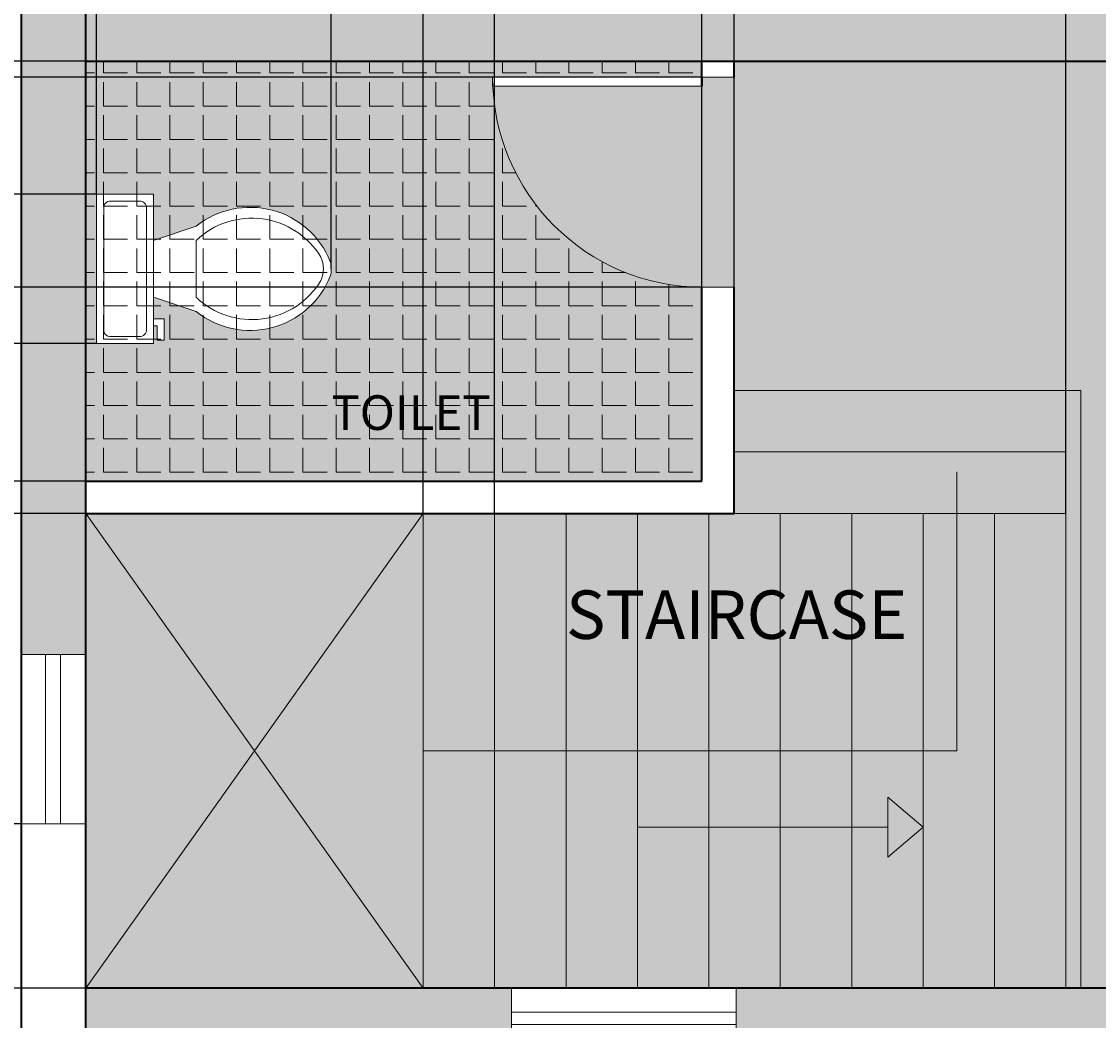
# Model space of a CAD drawing. Units: millimetres. Extents: x -229 to 16545, y -10488 to 4272.
# Tile 3 of 29: x 2016 to 5862, y -4633 to -1067. Entities that reach past the tile are written whole.
import ezdxf

# ---------------------------------------------------------------- set-up
doc = ezdxf.new("R2010")
doc.units = ezdxf.units.MM
for name, color, linetype, lineweight in [('A-ANNO-DIMS', 2, 'Continuous', 18), ('A-ANNO-SYMB', 7, 'Continuous', 18), ('A-AREA-IDEN', 7, 'Continuous', 18), ('A-DOOR', 4, 'Continuous', 18), ('A-FLOR-FIXT', 8, 'Continuous', 18), ('A-FLOR-PATT-TILE', 8, 'Continuous', 13), ('A-FLOR-STRS', 7, 'Continuous', 18), ('A-GLAZ', 4, 'Continuous', 18), ('A-WALL', 7, 'Continuous', 35)]:
    doc.layers.add(name, color=color, linetype=linetype, lineweight=lineweight)
for name, color, linetype, lineweight, true_color in [('A-FLOR-PATT', 254, 'Continuous', 13, 0xfeeab9), ('A-FLOR-STRS-PATT', 51, 'Continuous', 13, 0xf8f6b0), ('A-WALL-PATT', 18, 'Continuous', 13, 0x000000)]:
    doc.layers.add(name, color=color, linetype=linetype, lineweight=lineweight, true_color=true_color)
doc.styles.get("Standard").update_dxf_attribs({"font": 'arial.ttf'})
doc.dimstyles.get("Standard").update_dxf_attribs({"dimtxt": 0.18, "dimasz": 0.18, "dimexe": 0.18, "dimexo": 0.0625, "dimgap": 0.09, "dimtad": 0, "dimtih": 1, "dimtoh": 1, "dimdec": 4, "dimzin": 0, "dimdsep": 46, "dimtxsty": 'Standard', "dimcen": 0.09, "dimadec": 0, "dimazin": 0, "dimtfac": 1, "dimtdec": 4, "dimtofl": 0, "dimtmove": 0, "dimatfit": 3, "dimfxl": 1, "dimtolj": 1, "dimtzin": 0, "dimarcsym": 0})

# ---------------------------------------------------------------- blocks, each defined once
blk = doc.blocks.new('*U13')
at = {"transparency": 33554687}
for p, q in [((0, 0), (0, -6)), ((-40, 0), (-40, -6))]:
    blk.add_line(p, q, dxfattribs=at)
blk.add_lwpolyline([(0, 0), (0, 40), (-1.75, 40), (-1.75, 0)], close=True, dxfattribs=at)
blk.add_arc((0, 0), 40, 90, 180, dxfattribs=at)
blk = doc.blocks.new('*U16')
for p, q in [((9.5, -6), (9.5, -2)), ((-10, -8.5), (-8, -8.5)), ((-10, -9.5), (-10, -8.5)), ((-8, -8.5), (-8, -8)), ((-7, -8), (-7, -9.5)), ((-4, -8), (-6, -14)), ((4, -8), (6, -14)), ((-7, -9.5), (-10, -9.5)), ((4, -14), (-4, -14))]:
    blk.add_line(p, q)
blk.add_lwpolyline([(10.5, -8), (10.5, 0), (-10.5, 0), (-10.5, -8)], close=True)
for points in [[(8.5, -1), (-8.5, -1)], [(-9.5, -2), (-9.5, -6)], [(-8.5, -7), (8.5, -7)]]:
    blk.add_lwpolyline(points)
for centre, radius, start, end in [((-8.62, -1.88), 0.884, 81.8699, 188.1301), ((8.62, -1.88), 0.884, 351.8699, 98.1301), ((-8.62, -6.12), 0.884, 171.8699, 278.1301), ((8.62, -6.12), 0.884, 261.8699, 8.1301), ((3.52, -21.58), 12.17, 141.4691, 247.9714), ((4.2, -21.82), 11.33, 136.3677, 238.9468), ((-3.52, -21.58), 12.17, 292.0284, 38.5307), ((-4.2, -21.82), 11.33, 301.053, 43.6321), ((0, -27.88), 4, 245.7318, 294.2682), ((0, -29), 4, 254.8605, 285.1395)]:
    blk.add_arc(centre, radius, start, end)
blk = doc.blocks.new('WIN-802')
at = {"transparency": 33554687}
for p, q in [((0, 145), (0, 230)), ((802.3, 145), (802.3, 230)), ((0, 100.7), (0, 0)), ((802.3, 100.7), (802.3, 0))]:
    blk.add_line(p, q, dxfattribs=at)
blk.add_lwpolyline([(0, 145), (802.3, 145), (802.3, 100.7), (0, 100.7)], close=True, dxfattribs=at)
blk = doc.blocks.new('*D54')
at = {"layer": 'A-ANNO-DIMS', "color": 0, "lineweight": -2, "transparency": 16777216}
for p, q in [((2245.933029, -2708.209552), (2245.933029, 4271.65929)), ((2246.113029, 4271.47929), (3345.573029, 4271.47929)), ((4445.753029, 4271.47929), (3346.293029, 4271.47929)), ((4445.933029, -2708.209552), (4445.933029, 4271.65929))]:
    blk.add_line(p, q, dxfattribs=at)
at = {"layer": 'A-ANNO-DIMS', "color": 0, "transparency": 16777216}
for points in [[(2246.113029, 4271.50929), (2246.113029, 4271.44929), (2245.933029, 4271.47929)], [(4445.753029, 4271.50929), (4445.753029, 4271.44929), (4445.933029, 4271.47929)]]:
    blk.add_solid(points, dxfattribs=at)
at = {"layer": 'Defpoints', "color": 0, "transparency": 16777216}
for p in [(4445.933029, 4271.47929), (2245.933029, -2708.272052), (4445.933029, -2708.272052)]:
    blk.add_point(p, dxfattribs=at)
at = {"layer": 'A-ANNO-DIMS', "color": 0, "transparency": 16777216, "insert": (3345.933029, 4271.47929), "char_height": 0.18, "attachment_point": 5}
blk.add_mtext('\\A1;2200', dxfattribs=at)
blk = doc.blocks.new('*D55')
at = {"layer": 'A-ANNO-DIMS', "color": 0, "lineweight": -2, "transparency": 16777216}
for p, q in [((4445.9, -1208.3), (-228.8, -1208.3)), ((-228.7, -1208.5), (-228.7, -1958.1)), ((-228.7, -2708.1), (-228.7, -1958.5)), ((4445.9, -2708.3), (-228.8, -2708.3))]:
    blk.add_line(p, q, dxfattribs=at)
at = {"layer": 'A-ANNO-DIMS', "color": 0, "transparency": 16777216}
for points in [[(-228.7, -1208.5), (-228.6, -1208.5), (-228.7, -1208.3)], [(-228.7, -2708.1), (-228.6, -2708.1), (-228.7, -2708.3)]]:
    blk.add_solid(points, dxfattribs=at)
at = {"layer": 'Defpoints', "color": 0, "transparency": 16777216}
for p in [(4445.9, -1208.3), (-228.7, -2708.3), (4445.9, -2708.3)]:
    blk.add_point(p, dxfattribs=at)
at = {"layer": 'A-ANNO-DIMS', "color": 0, "transparency": 16777216, "insert": (-228.7, -1958.3), "char_height": 0.18, "attachment_point": 5}
blk.add_mtext('\\A1;1500', dxfattribs=at)
blk = doc.blocks.new('*D56')
at = {"layer": 'A-ANNO-DIMS', "color": 0, "lineweight": -2, "transparency": 16777216}
for p, q in [((2245.9, -2823.3), (-228.8, -2823.3)), ((-228.7, -2823.5), (-228.7, -3670.6)), ((-228.7, -4518.1), (-228.7, -3671)), ((2245.9, -4518.3), (-228.8, -4518.3))]:
    blk.add_line(p, q, dxfattribs=at)
at = {"layer": 'A-ANNO-DIMS', "color": 0, "transparency": 16777216}
for points in [[(-228.7, -2823.5), (-228.6, -2823.5), (-228.7, -2823.3)], [(-228.7, -4518.1), (-228.6, -4518.1), (-228.7, -4518.3)]]:
    blk.add_solid(points, dxfattribs=at)
at = {"layer": 'Defpoints', "color": 0, "transparency": 16777216}
for p in [(2245.9, -2823.3), (-228.7, -4518.3), (2245.9, -4518.3)]:
    blk.add_point(p, dxfattribs=at)
at = {"layer": 'A-ANNO-DIMS', "color": 0, "transparency": 16777216, "insert": (-228.7, -3670.8), "char_height": 0.18, "attachment_point": 5}
blk.add_mtext('\\A1;1695', dxfattribs=at)
blk = doc.blocks.new('*D81')
at = {"layer": 'A-ANNO-DIMS', "color": 0, "lineweight": -2, "transparency": 16777216}
for p, q in [((2245.9, -2823.2), (2245.9, 4271.7)), ((2246.1, 4271.5), (2847.7, 4271.5)), ((3450.2, 4271.5), (2848.6, 4271.5)), ((3450.4, -2823.2), (3450.4, 4271.7))]:
    blk.add_line(p, q, dxfattribs=at)
at = {"layer": 'A-ANNO-DIMS', "color": 0, "transparency": 16777216}
for points in [[(2246.1, 4271.5), (2246.1, 4271.4), (2245.9, 4271.5)], [(3450.2, 4271.5), (3450.2, 4271.4), (3450.4, 4271.5)]]:
    blk.add_solid(points, dxfattribs=at)
at = {"layer": 'Defpoints', "color": 0, "transparency": 16777216}
for p in [(3450.4, 4271.5), (2245.9, -2823.3), (3450.4, -2823.3)]:
    blk.add_point(p, dxfattribs=at)
at = {"layer": 'A-ANNO-DIMS', "color": 0, "transparency": 16777216, "insert": (2848.2, 4271.5), "char_height": 0.18, "attachment_point": 5}
blk.add_mtext('\\A1;1204.5', dxfattribs=at)
blk = doc.blocks.new('*D82')
at = {"layer": 'A-ANNO-DIMS', "color": 0, "lineweight": -2, "transparency": 16777216}
for p, q in [((3450.4, -2823.2), (3450.4, 4271.7)), ((3450.6, 4271.5), (3577.5, 4271.5)), ((3705.3, 4271.5), (3578.4, 4271.5)), ((3705.5, -2823.2), (3705.5, 4271.7))]:
    blk.add_line(p, q, dxfattribs=at)
at = {"layer": 'A-ANNO-DIMS', "color": 0, "transparency": 16777216}
for points in [[(3450.6, 4271.5), (3450.6, 4271.4), (3450.4, 4271.5)], [(3705.3, 4271.5), (3705.3, 4271.4), (3705.5, 4271.5)]]:
    blk.add_solid(points, dxfattribs=at)
at = {"layer": 'Defpoints', "color": 0, "transparency": 16777216}
for p in [(3705.5, 4271.5), (3450.4, -2823.3), (3705.5, -2823.3)]:
    blk.add_point(p, dxfattribs=at)
at = {"layer": 'A-ANNO-DIMS', "color": 0, "transparency": 16777216, "insert": (3577.9, 4271.5), "char_height": 0.18, "attachment_point": 5}
blk.add_mtext('\\A1;255.06', dxfattribs=at)
blk = doc.blocks.new('*D83')
at = {"layer": 'A-ANNO-DIMS', "color": 0, "lineweight": -2, "transparency": 16777216}
for p, q in [((4448.4, -1265.8), (-228.8, -1265.8)), ((-228.7, -1266), (-228.7, -1640.6)), ((-228.7, -2015.6), (-228.7, -1641)), ((4445.9, -2015.8), (-228.8, -2015.8))]:
    blk.add_line(p, q, dxfattribs=at)
at = {"layer": 'A-ANNO-DIMS', "color": 0, "transparency": 16777216}
for points in [[(-228.7, -1266), (-228.6, -1266), (-228.7, -1265.8)], [(-228.7, -2015.6), (-228.6, -2015.6), (-228.7, -2015.8)]]:
    blk.add_solid(points, dxfattribs=at)
at = {"layer": 'Defpoints', "color": 0, "transparency": 16777216}
for p in [(4448.4, -1265.8), (-228.7, -2015.8), (4445.9, -2015.8)]:
    blk.add_point(p, dxfattribs=at)
at = {"layer": 'A-ANNO-DIMS', "color": 0, "transparency": 16777216, "insert": (-228.7, -1640.8), "char_height": 0.18, "attachment_point": 5}
blk.add_mtext('\\A1;750', dxfattribs=at)
blk = doc.blocks.new('*D84')
at = {"layer": 'A-ANNO-DIMS', "color": 0, "lineweight": -2, "transparency": 16777216}
for p, q in [((4445.9, -2708.2), (4445.9, 4271.7)), ((4446.1, 4271.5), (4503.2, 4271.5)), ((4560.8, 4271.5), (4503.7, 4271.5)), ((4560.9, -2823.2), (4560.9, 4271.7))]:
    blk.add_line(p, q, dxfattribs=at)
at = {"layer": 'A-ANNO-DIMS', "color": 0, "transparency": 16777216}
for points in [[(4446.1, 4271.5), (4446.1, 4271.4), (4445.9, 4271.5)], [(4560.8, 4271.5), (4560.8, 4271.4), (4560.9, 4271.5)]]:
    blk.add_solid(points, dxfattribs=at)
at = {"layer": 'Defpoints', "color": 0, "transparency": 16777216}
for p in [(4560.9, 4271.5), (4445.9, -2708.3), (4560.9, -2823.3)]:
    blk.add_point(p, dxfattribs=at)
at = {"layer": 'A-ANNO-DIMS', "color": 0, "transparency": 16777216, "insert": (4503.4, 4271.5), "char_height": 0.18, "attachment_point": 5}
blk.add_mtext('\\A1;115', dxfattribs=at)
blk = doc.blocks.new('*D88')
at = {"layer": 'A-ANNO-DIMS', "color": 0, "lineweight": -2, "transparency": 16777216}
for p, q in [((2015.9, -3931), (-228.8, -3931)), ((-228.7, -3931.2), (-228.7, -4224.5)), ((-228.7, -4518.1), (-228.7, -4224.8)), ((2245.9, -4518.3), (-228.8, -4518.3))]:
    blk.add_line(p, q, dxfattribs=at)
at = {"layer": 'A-ANNO-DIMS', "color": 0, "transparency": 16777216}
for points in [[(-228.7, -3931.2), (-228.6, -3931.2), (-228.7, -3931)], [(-228.7, -4518.1), (-228.6, -4518.1), (-228.7, -4518.3)]]:
    blk.add_solid(points, dxfattribs=at)
at = {"layer": 'Defpoints', "color": 0, "transparency": 16777216}
for p in [(2015.9, -3931), (-228.7, -4518.3), (2245.9, -4518.3)]:
    blk.add_point(p, dxfattribs=at)
at = {"layer": 'A-ANNO-DIMS', "color": 0, "transparency": 16777216, "insert": (-228.7, -4224.7), "char_height": 0.18, "attachment_point": 5}
blk.add_mtext('\\A1;587.2', dxfattribs=at)
blk = doc.blocks.new('*D93')
at = {"layer": 'A-ANNO-DIMS', "color": 0, "lineweight": -2, "transparency": 16777216}
for p, q in [((2284, -1683.4), (2284, 4271.7)), ((2284.2, 4271.5), (2702.7, 4271.5)), ((3122, 4271.5), (2703.5, 4271.5)), ((3122.2, -1950.1), (3122.2, 4271.7))]:
    blk.add_line(p, q, dxfattribs=at)
at = {"layer": 'A-ANNO-DIMS', "color": 0, "transparency": 16777216}
for points in [[(2284.2, 4271.5), (2284.2, 4271.4), (2284, 4271.5)], [(3122, 4271.5), (3122, 4271.4), (3122.2, 4271.5)]]:
    blk.add_solid(points, dxfattribs=at)
at = {"layer": 'Defpoints', "color": 0, "transparency": 16777216}
for p in [(3122.2, 4271.5), (2284, -1683.5), (3122.2, -1950.2)]:
    blk.add_point(p, dxfattribs=at)
at = {"layer": 'A-ANNO-DIMS', "color": 0, "transparency": 16777216, "insert": (2703.1, 4271.5), "char_height": 0.18, "attachment_point": 5}
blk.add_mtext('\\A1;838.2', dxfattribs=at)
blk = doc.blocks.new('*D94')
at = {"layer": 'A-ANNO-DIMS', "color": 0, "lineweight": -2, "transparency": 16777216}
for p, q in [((2283.9, -1683.5), (-228.8, -1683.5)), ((-228.7, -1683.7), (-228.7, -1950)), ((-228.7, -2216.7), (-228.7, -1950.4)), ((2283.9, -2216.9), (-228.8, -2216.9))]:
    blk.add_line(p, q, dxfattribs=at)
at = {"layer": 'A-ANNO-DIMS', "color": 0, "transparency": 16777216}
for points in [[(-228.7, -1683.7), (-228.6, -1683.7), (-228.7, -1683.5)], [(-228.7, -2216.7), (-228.6, -2216.7), (-228.7, -2216.9)]]:
    blk.add_solid(points, dxfattribs=at)
at = {"layer": 'Defpoints', "color": 0, "transparency": 16777216}
for p in [(2284, -1683.5), (-228.7, -2216.9), (2284, -2216.9)]:
    blk.add_point(p, dxfattribs=at)
at = {"layer": 'A-ANNO-DIMS', "color": 0, "transparency": 16777216, "insert": (-228.7, -1950.2), "char_height": 0.18, "attachment_point": 5}
blk.add_mtext('\\A1;533.4', dxfattribs=at)
blk = doc.blocks.new('*D97')
at = {"layer": 'A-ANNO-DIMS', "color": 0, "lineweight": -2, "transparency": 16777216}
for p, q in [((3450.4, -2823.2), (3450.4, 4271.7)), ((3450.6, 4271.5), (4597.7, 4271.5)), ((5745.8, 4271.5), (4598.6, 4271.5)), ((5745.9, -2823.2), (5745.9, 4271.7))]:
    blk.add_line(p, q, dxfattribs=at)
at = {"layer": 'A-ANNO-DIMS', "color": 0, "transparency": 16777216}
for points in [[(3450.6, 4271.5), (3450.6, 4271.4), (3450.4, 4271.5)], [(5745.8, 4271.5), (5745.8, 4271.4), (5745.9, 4271.5)]]:
    blk.add_solid(points, dxfattribs=at)
at = {"layer": 'Defpoints', "color": 0, "transparency": 16777216}
for p in [(5745.9, 4271.5), (3450.4, -2823.3), (5745.9, -2823.3)]:
    blk.add_point(p, dxfattribs=at)
at = {"layer": 'A-ANNO-DIMS', "color": 0, "transparency": 16777216, "insert": (4598.2, 4271.5), "char_height": 0.18, "attachment_point": 5}
blk.add_mtext('\\A1;2295.5', dxfattribs=at)

msp = doc.modelspace()

# ---------------------------------------------------------------- hatches: boundary and pattern name
at = {"layer": 'A-ANNO-SYMB', "transparency": 33554615}
h = msp.add_hatch(color=256, dxfattribs=at)
h.dxf.hatch_style = 1
h.paths.add_polyline_path([(5109.521, -3836.564), (5109.521, -4050.631), (5235.818, -3943.598)])
at = {"layer": 'A-FLOR-PATT', "transparency": 33554592}
h = msp.add_hatch(color=256, dxfattribs=at)
h.dxf.hatch_style = 1
h.paths.add_polyline_path([(7975.933, -5325.772), (7943.121, -5325.772), (7943.121, -4576.49, 0.40145271), (7225.933, -5325.772, 0.40145271), (6508.746, -4576.49), (6508.746, -5325.772), (6475.933, -5325.772), (6475.933, -5438.272), (5975.933, -5438.272), (5975.933, -7267.724), (5975.933, -7438.272), (6478.619, -7438.272), (6463.448, -7355.919), (6464.88, -7356.837), (6463.849, -7358.097), (6478.619, -7438.272), (6610.327, -7438.272), (6632.656, -7409.564), (6632.525, -7406.967), (6634.208, -7407.569), (6619.273, -7426.77), (6654.466, -7438.272), (7610.517, -7438.272), (7607.41, -7421.409), (7608.842, -7422.327), (7607.812, -7423.587), (7610.517, -7438.272), (7975.933, -7438.272)])
h.paths.add_polyline_path([(13785.933, -1208.272), (9555.933, -1208.272), (9555.933, -961.785), (9705.933, -961.785), (9705.933, -918.035), (10704.976, -918.035, 0.40145271), (9705.933, 38.215), (9555.933, 38.215), (9555.933, 2021.728), (5975.933, 2021.728), (5975.933, 755.492), (5745.933, 755.492), (5745.933, 1427.266), (2918.813, 1427.266), (2918.813, -492.942), (5013.319, -492.942), (5013.319, -978.272), (5745.933, -978.272), (5745.933, -397.513), (5975.933, -397.513), (5975.933, -1208.272), (4560.933, -1208.272), (4560.933, -1265.772), (4448.433, -1265.772), (4448.433, -1298.585), (4445.933, -1298.585), (3699.151, -1298.585, 0.40145271), (4448.433, -2015.772), (4560.933, -2015.772), (4560.933, -2384.177), (5745.933, -2384.177), (5799.402, -2384.177), (5799.402, -4518.272), (5975.933, -4518.272), (5975.933, -5208.272), (6475.933, -5208.272), (6475.933, -4575.772), (6508.746, -4575.772), (6508.746, -4576.49, -0.35647263), (7216.672, -5208.272), (7235.194, -5208.272, -0.35647263), (7943.121, -4576.49), (7943.121, -4575.772), (7975.933, -4575.772), (7975.933, -5208.272), (11176.247, -5208.272), (11159.44, -5191.465), (10520.768, -5191.465), (10520.768, -4888.936), (10571.19, -4888.936), (10571.19, -4872.129), (10772.876, -4872.129), (10772.876, -4888.936), (10789.683, -4888.936), (10789.683, -4872.129), (10991.368, -4872.129), (10991.368, -4888.936), (11041.79, -4888.936), (11041.79, -4872.129), (11058.597, -4872.129, -0.09090909), (11428.354, -4872.129), (11445.162, -4872.129), (11445.162, -4888.936), (11529.197, -4888.936), (11529.197, -5191.465), (11327.512, -5191.465), (11310.704, -5208.272), (13785.933, -5208.272)])
h.paths.add_polyline_path([(11047.216, -1630.944, -1), (11402.816, -1630.944, -1)], flags=16)
h.paths.add_polyline_path([(11148.816, -1630.944), (11225.016, -1554.744), (11301.216, -1630.944), (11225.016, -1707.144)], flags=0)
h.paths.add_polyline_path([(11199.616, -1630.944, -1), (11250.416, -1630.944, -1)], flags=0)
h.paths.add_polyline_path([(11588.751, -2096.259), (11588.751, -1543.254, -0.26666697), (12864.918, -1543.254), (12864.918, -2096.259), (12737.302, -2096.259), (12737.302, -2063.121), (11716.368, -2063.121), (11716.368, -2096.259)], flags=16)
h.paths.add_polyline_path([(12012.696, -2489.42), (12600.997, -2489.42), (12600.997, -3666.022), (12012.696, -3666.022)], flags=16)
h.paths.add_polyline_path([(12176.41, -3599.403), (12174.938, -3609.076), (12173.789, -3618.819), (12173.09, -3628.559), (12172.973, -3638.221), (12173.89, -3652.852), (12175.008, -3657.025), (12172.909, -3643.473), (12173.142, -3624.297), (12175.386, -3605.273)], flags=0)
h.paths.add_polyline_path([(8026.289, -286.944), (7737.703, -287.19), (7734.87, -269.156), (8029.092, -268.905)], flags=16)
h.paths.add_polyline_path([(7733.453, -260.139), (7710.784, -115.865), (7557.191, -115.996), (7556.999, 109.744), (7412.687, 132.166), (7412.433, 429.206), (7556.707, 451.876), (7556.568, 614.769), (7412.256, 637.19), (7412.003, 934.231), (7556.276, 956.9), (7556.084, 1182.639), (7709.677, 1182.77), (7732.099, 1327.082), (8029.14, 1327.335), (8051.808, 1183.062), (8205.401, 1183.192), (8205.594, 957.454), (8349.906, 935.031), (8350.159, 637.99), (8205.885, 615.322), (8206.024, 452.43), (8350.336, 430.006), (8350.59, 132.965), (8206.316, 110.298), (8206.509, -115.442), (8052.916, -115.573), (8030.493, -259.885)], flags=16)
h.paths.add_polyline_path([(12261.416, -3475.554), (12262.632, -3486.776), (12264.032, -3497.007), (12265.554, -3506.365), (12267.136, -3514.968), (12268.719, -3522.935), (12271.304, -3535.59), (12273.606, -3548.078), (12275.271, -3561.064), (12275.93, -3574.938), (12275.325, -3590.3), (12273.425, -3607.964), (12270.795, -3625.658), (12268.066, -3641.063), (12266.318, -3649.679), (12265.456, -3653.626), (12263.984, -3659.846), (12264.032, -3659.566), (12264.342, -3658.241), (12264.807, -3656.37), (12265.456, -3653.626), (12266.318, -3649.679), (12267.409, -3644.302), (12268.668, -3637.664), (12270.019, -3630.037), (12271.384, -3621.695), (12272.69, -3612.908), (12273.857, -3603.948), (12274.81, -3595.088), (12275.47, -3586.601), (12275.782, -3578.689), (12275.757, -3571.292), (12275.423, -3564.275), (12274.816, -3557.512), (12273.964, -3550.872), (12272.896, -3544.224), (12271.645, -3537.439), (12270.24, -3530.385), (12267.543, -3517.181), (12264.612, -3501.247), (12261.849, -3481.059)], flags=0)
h.paths.add_polyline_path([(12332.136, -3408.03), (12333.483, -3416.79), (12335.077, -3424.54), (12336.915, -3431.355), (12338.991, -3437.32), (12341.266, -3442.55), (12343.694, -3447.166), (12346.229, -3451.292), (12348.826, -3455.051), (12351.438, -3458.563), (12357.476, -3466.491), (12363.61, -3476.575), (12368.309, -3489.762), (12369.929, -3503.427), (12369.842, -3516.511), (12368.43, -3530.867), (12365.816, -3545.835), (12362.382, -3559.786), (12360.968, -3564.487), (12363.063, -3557.021), (12364.898, -3549.566), (12366.473, -3542.077), (12367.773, -3534.631), (12368.781, -3527.301), (12369.483, -3520.162), (12369.863, -3513.291), (12369.906, -3506.759), (12369.599, -3500.643), (12368.93, -3494.999), (12367.924, -3489.796), (12366.61, -3484.994), (12365.024, -3480.542), (12363.19, -3476.399), (12361.141, -3472.516), (12358.909, -3468.847), (12356.525, -3465.347), (12354.02, -3461.954), (12351.438, -3458.563), (12345.462, -3450.529), (12339.923, -3439.996), (12335.85, -3428.296), (12332.68, -3412.888)], flags=0)
h.paths.add_polyline_path([(12385.287, -3334.612), (12384.977, -3342.409), (12385.02, -3349.196), (12385.4, -3355.066), (12386.104, -3360.105), (12387.112, -3364.41), (12388.412, -3368.071), (12389.987, -3371.181), (12391.823, -3373.832), (12393.919, -3376.097), (12396.337, -3377.978), (12399.153, -3379.462), (12402.445, -3380.531), (12406.289, -3381.172), (12410.758, -3381.371), (12415.935, -3381.106), (12421.893, -3380.368), (12428.658, -3379.159), (12436.069, -3377.55), (12443.907, -3375.635), (12451.961, -3373.505), (12460.015, -3371.254), (12467.853, -3368.971), (12475.263, -3366.749), (12482.029, -3364.68), (12491.877, -3361.657), (12497.701, -3360.107), (12501.639, -3359.288), (12510.135, -3358.326), (12519.662, -3365.412), (12524.243, -3378.911), (12523.764, -3390.7), (12520.746, -3401.577), (12514.248, -3415.634), (12511.518, -3420.418), (12515.856, -3412.154), (12519.153, -3405.024), (12521.516, -3398.804), (12523.049, -3393.276), (12523.865, -3388.212), (12524.059, -3383.441), (12523.7, -3378.958), (12522.853, -3374.815), (12521.576, -3371.054), (12519.931, -3367.722), (12517.982, -3364.865), (12515.786, -3362.529), (12513.405, -3360.758), (12510.877, -3359.588), (12508.136, -3358.982), (12505.086, -3358.897), (12501.639, -3359.288), (12497.701, -3360.107), (12493.183, -3361.309), (12487.988, -3362.851), (12476.403, -3366.408), (12463.335, -3370.326), (12447.372, -3374.788), (12431.759, -3378.604), (12418.504, -3380.974), (12405.811, -3381.624), (12394.725, -3378.025), (12388.039, -3368.367), (12385.583, -3357.877), (12384.826, -3346.204), (12385.428, -3331.059), (12385.953, -3325.719)], flags=0)
h.paths.add_polyline_path([(7880.016, 1173.969), (7880.373, 1175.495), (7880.433, 1175.851), (7879.484, 1171.818)], flags=0)
h.paths.add_polyline_path([(7802.33, 874.962), (7800.771, 885.032), (7798.932, 893.941), (7796.811, 901.774), (7794.419, 908.63), (7791.798, 914.639), (7789.002, 919.945), (7786.083, 924.686), (7783.093, 929.005), (7780.087, 933.043), (7774.996, 939.717), (7768.406, 949.37), (7762.174, 963.427), (7759.342, 978.002), (7758.629, 991.888), (7759.492, 1007.928), (7761.801, 1025.496), (7765.392, 1044.035), (7766.625, 1049.048), (7764.522, 1039.543), (7762.719, 1030.232), (7761.232, 1021.168), (7760.08, 1012.405), (7759.28, 1003.994), (7758.849, 995.988), (7758.806, 988.44), (7759.167, 981.404), (7759.942, 974.914), (7761.104, 968.936), (7762.617, 963.414), (7764.448, 958.299), (7766.559, 953.535), (7768.918, 949.073), (7771.487, 944.856), (7774.232, 940.835), (7777.115, 936.938), (7782.377, 930.041), (7787.845, 922.139), (7793.348, 911.698), (7798.042, 898.247), (7801.702, 880.527)], flags=0)
h.paths.add_polyline_path([(12519.068, -3228.534), (12519.615, -3236.235), (12520.529, -3242.343), (12521.78, -3247.103), (12523.337, -3250.758), (12525.171, -3253.556), (12527.248, -3255.709), (12529.522, -3257.296), (12531.95, -3258.361), (12534.486, -3258.949), (12537.082, -3259.11), (12539.694, -3258.888), (12542.277, -3258.329), (12544.781, -3257.478), (12547.173, -3256.388), (12549.46, -3255.129), (12550.455, -3254.517), (12555.825, -3251.109), (12557.835, -3249.942), (12565.181, -3246.404), (12574.565, -3253.032), (12576.931, -3265.022), (12576.627, -3277.425), (12575.416, -3290.819), (12574.851, -3295.392), (12575.708, -3287.593), (12576.322, -3280.806), (12576.688, -3274.939), (12576.812, -3269.899), (12576.688, -3265.593), (12576.322, -3261.932), (12575.708, -3258.822), (12574.851, -3256.172), (12573.753, -3253.905), (12572.439, -3252.005), (12570.943, -3250.474), (12569.293, -3249.309), (12567.523, -3248.513), (12565.658, -3248.083), (12563.732, -3248.022), (12561.777, -3248.328), (12559.814, -3248.989), (12557.835, -3249.942), (12555.825, -3251.109), (12553.77, -3252.413), (12551.652, -3253.78), (12549.46, -3255.129), (12543.167, -3258.594), (12532.661, -3259.485), (12524.685, -3253.923), (12520.949, -3245.152), (12519.138, -3233.042)], flags=0)
h.paths.add_polyline_path([(7741.293, 790.501), (7741.641, 799.467), (7741.584, 807.269), (7741.141, 814.015), (7740.329, 819.809), (7739.165, 824.757), (7737.667, 828.966), (7735.853, 832.541), (7733.74, 835.586), (7731.348, 838.188), (7728.71, 840.348), (7725.861, 842.052), (7722.836, 843.28), (7719.671, 844.015), (7716.4, 844.237), (7713.06, 843.932), (7709.684, 843.081), (7706.304, 841.686), (7702.923, 839.834), (7699.543, 837.629), (7696.164, 835.178), (7692.784, 832.585), (7684.718, 826.315), (7675.609, 820.63), (7664.001, 817.274), (7654.105, 821.884), (7647.171, 832.02), (7644.191, 846.522), (7646.321, 860.288), (7647.49, 864.223), (7645.946, 857.865), (7645.046, 852.044), (7644.827, 846.557), (7645.243, 841.404), (7646.221, 836.642), (7647.693, 832.318), (7649.587, 828.489), (7651.832, 825.206), (7654.359, 822.523), (7657.097, 820.49), (7659.984, 819.145), (7662.993, 818.452), (7666.108, 818.357), (7669.311, 818.809), (7672.583, 819.755), (7675.908, 821.139), (7679.268, 822.913), (7682.645, 825.021), (7686.025, 827.401), (7689.404, 829.958), (7692.784, 832.585), (7700.505, 838.509), (7709.871, 843.64), (7721.436, 844.698), (7733.277, 837.617), (7739.571, 825.214), (7741.557, 811.049), (7741.669, 795.575)], flags=0)
h.paths.add_polyline_path([(8377.641, 137.216), (8359.607, 134.382), (8359.356, 428.605), (8377.395, 425.802)], flags=16)
h.paths.add_polyline_path([(7650.715, 668.465), (7650.08, 677.319), (7649.023, 684.34), (7647.579, 689.811), (7645.785, 694.012), (7643.675, 697.228), (7641.286, 699.7), (7638.669, 701.521), (7635.876, 702.744), (7632.96, 703.419), (7629.974, 703.601), (7626.971, 703.344), (7624.004, 702.697), (7621.125, 701.717), (7618.375, 700.462), (7615.749, 699.013), (7614.561, 698.279), (7608.435, 694.382), (7606.125, 693.04), (7598.981, 689.594), (7589.669, 693.773), (7585.26, 702.856), (7584.221, 713.11), (7584.49, 724.584), (7585.863, 739.937), (7586.518, 745.277), (7585.539, 736.31), (7584.841, 728.507), (7584.424, 721.761), (7584.288, 715.966), (7584.433, 711.016), (7584.86, 706.807), (7585.567, 703.231), (7586.556, 700.186), (7587.821, 697.58), (7589.332, 695.397), (7591.053, 693.637), (7592.951, 692.3), (7594.989, 691.385), (7597.132, 690.895), (7599.346, 690.826), (7601.594, 691.18), (7603.851, 691.943), (7606.125, 693.04), (7608.435, 694.382), (7610.797, 695.885), (7613.229, 697.458), (7620.475, 701.929), (7632.001, 704.44), (7643.476, 699.417), (7648.536, 687.571), (7650.63, 673.661)], flags=0)
h.paths.add_polyline_path([(7385.628, 136.37), (7385.382, 424.956), (7403.416, 427.789), (7403.667, 133.567)], flags=16)
h.paths.add_polyline_path([(12993.884, -2257.186), (12959.588, -2257.186), (12959.588, -2125.099), (13531.966, -2125.099, -0.19047621), (13531.966, -3974.321), (12959.588, -3974.321), (12959.588, -3842.233), (12993.884, -3842.233)], flags=16)
h.paths.add_polyline_path([(13413.486, -3313.884), (13413.486, -2785.535), (13562.885, -2785.535, -0.04962821), (13562.885, -3313.884)], flags=0)
h.paths.add_polyline_path([(8377.21, 642.241), (8359.176, 639.407), (8358.925, 933.629), (8376.964, 930.826)], flags=16)
h.paths.add_polyline_path([(13086.058, -1864.83), (13086.058, -1449.84), (13501.048, -1449.84), (13501.048, -1864.83)], flags=16)
h.paths.add_polyline_path([(13305.814, -1862.197), (13302.103, -1859.624), (13298.088, -1857.068), (13293.799, -1854.536), (13289.262, -1852.031), (13284.504, -1849.559), (13279.554, -1847.125), (13274.439, -1844.735), (13269.17, -1842.389), (13263.701, -1840.081), (13257.97, -1837.797), (13251.914, -1835.525), (13245.472, -1833.252), (13238.582, -1830.968), (13231.18, -1828.66), (13223.206, -1826.315), (13209.182, -1822.458), (13204.584, -1821.48), (13217.962, -1824.773), (13235.072, -1829.804), (13248.777, -1834.349), (13260.829, -1838.869), (13274.479, -1844.63), (13289.675, -1852.101), (13302.553, -1859.704)], flags=0)
h.paths.add_polyline_path([(13428.104, -1820.994), (13419.007, -1818.141), (13409.95, -1815.4), (13400.766, -1812.747), (13391.271, -1810.151), (13376.087, -1806.251), (13370.618, -1805.019), (13386.304, -1808.794), (13405.087, -1813.928), (13423.014, -1819.354)], flags=0)
h.paths.add_polyline_path([(7385.197, 641.395), (7384.951, 929.98), (7402.986, 932.814), (7403.236, 638.592)], flags=16)
h.paths.add_polyline_path([(13262.537, -1725.526), (13253.246, -1724.74), (13244.516, -1724.117), (13235.94, -1723.625), (13223.267, -1723.062), (13217.598, -1722.912), (13231.966, -1723.397), (13248.733, -1724.359), (13266.899, -1725.895), (13272.802, -1726.502)], flags=0)
h.paths.add_polyline_path([(13191.893, -1641.137), (13208.675, -1640.506), (13214.057, -1640.258), (13197.763, -1640.936)], flags=0)
h.paths.add_polyline_path([(13097.524, -1608.457), (13114.284, -1609.031), (13120.126, -1609.105), (13103.045, -1608.71)], flags=0)
h.paths.add_polyline_path([(13465.328, -1521.577), (13473.906, -1517.015), (13481.761, -1511.636), (13492.562, -1502.076), (13495.327, -1497.933), (13485.818, -1508.858), (13470.208, -1519.547)], flags=0)
h.paths.add_polyline_path([(13175.015, -1500.891), (13184.046, -1501.807), (13192.721, -1502.52), (13201.114, -1503.034), (13209.273, -1503.351), (13217.244, -1503.476), (13225.078, -1503.41), (13232.821, -1503.16), (13240.524, -1502.728), (13248.233, -1502.117), (13255.993, -1501.322), (13263.825, -1500.293), (13271.746, -1498.974), (13279.775, -1497.305), (13287.928, -1495.229), (13296.222, -1492.688), (13304.675, -1489.622), (13313.304, -1485.975), (13322.089, -1481.727), (13330.859, -1477.028), (13339.408, -1472.063), (13347.526, -1467.02), (13355.006, -1462.087), (13364.86, -1455.202), (13367.224, -1453.299), (13358.544, -1459.754), (13343.348, -1469.775), (13326.143, -1479.767), (13309.023, -1488.045), (13292.249, -1494.129), (13276.009, -1498.264), (13260.299, -1500.88), (13244.401, -1502.51), (13228.945, -1503.378), (13213.316, -1503.508), (13197.047, -1502.876), (13180.088, -1501.481)], flags=0)
h.paths.add_polyline_path([(7733.501, 1336.101), (7736.303, 1354.14), (8024.889, 1354.386), (8027.723, 1336.352)], flags=16)
at = {"layer": 'A-FLOR-PATT', "transparency": 33554534}
h = msp.add_hatch(color=256, dxfattribs=at)
h.dxf.hatch_style = 1
h.paths.add_polyline_path([(4445.933, -2015.768, -0.4004854), (3699.151, -1298.585), (3698.433, -1298.585), (3698.433, -1265.772), (4445.933, -1265.772), (4445.933, -1208.272), (2245.933, -1208.272), (2245.933, -2708.272), (4445.933, -2708.272)])
h.paths.add_polyline_path([(3118.674, -1976.734, -0.50131678), (2639.604, -2102.6), (2487.202, -2051.799), (2487.202, -2127.999), (2525.302, -2127.999), (2525.302, -2204.199), (2499.902, -2204.199), (2499.902, -2153.399), (2487.202, -2153.399), (2487.202, -2216.899), (2284.002, -2216.899), (2284.002, -1683.499), (2487.202, -1683.499), (2487.202, -1848.599), (2639.599, -1797.8, -0.50132349), (3118.674, -1923.664, -0.13289091)], flags=16)
h.paths.add_polyline_path([(3084.686, -1991.957, -0.48007965), (2639.602, -2051.798), (2639.602, -1848.598, -0.4800795), (3084.686, -1908.44, -0.21500378)], flags=0)
h.paths.add_polyline_path([(2461.802, -2166.099, -0.41421356), (2442.752, -2191.499), (2334.802, -2191.499, -0.41421356), (2309.402, -2172.449), (2309.402, -1734.299, -0.41421356), (2328.452, -1708.899), (2436.402, -1708.899, -0.41421356), (2461.802, -1727.949)], flags=0)
at = {"layer": 'A-FLOR-PATT-TILE', "transparency": 33554493}
h = msp.add_hatch(dxfattribs=at)
h.set_pattern_fill('ANGLE', color=256, scale=17)
h.set_pattern_definition([(0, (-8141.22, -13125.5), (0, 118.745), [86.36, -32.385]), (90, (-8141.22, -13125.5), (-118.745, 7e-15), [86.36, -32.385])])
h.paths.add_polyline_path([(4445.933, -2015.768, -0.4004854), (3699.151, -1298.585), (3698.433, -1298.585), (3698.433, -1265.772), (4445.933, -1265.772), (4445.933, -1208.272), (2245.933, -1208.272), (2245.933, -2708.272), (4445.933, -2708.272)])
at = {"layer": 'A-FLOR-STRS-PATT', "transparency": 33554615}
h = msp.add_hatch(color=256, dxfattribs=at)
h.dxf.hatch_style = 1
h.paths.add_polyline_path([(3450.417, -2823.272), (2848.175, -3670.772), (3450.417, -4518.272)])
h.paths.add_polyline_path([(2848.175, -3670.772), (2245.933, -4518.272), (3450.417, -4518.272)])
h.paths.add_polyline_path([(2245.933, -2823.272), (2245.933, -4518.272), (2848.175, -3670.772)])
h.paths.add_polyline_path([(3450.417, -2823.272), (2245.933, -2823.272), (2848.175, -3670.772)])
h.paths.add_polyline_path([(3705.475, -2823.272), (3450.417, -2823.272), (3450.417, -3670.772), (3705.475, -3670.772)])
h.paths.add_polyline_path([(3960.532, -2823.272), (3705.475, -2823.272), (3705.475, -3670.772), (3960.532, -3670.772)])
h.paths.add_polyline_path([(4215.589, -2823.272), (3960.532, -2823.272), (3960.532, -3670.772), (4215.589, -3670.772)])
h.paths.add_polyline_path([(4470.646, -2823.272), (4215.589, -2823.272), (4215.589, -3670.772), (4470.646, -3670.772)])
h.paths.add_polyline_path([(4725.704, -2823.272), (4560.933, -2823.272), (4470.646, -2823.272), (4470.646, -3670.772), (4725.704, -3670.772)])
h.paths.add_polyline_path([(4980.761, -2823.272), (4725.704, -2823.272), (4725.704, -3670.772), (4980.761, -3670.772)])
h.paths.add_polyline_path([(5235.818, -2823.272), (4980.761, -2823.272), (4980.761, -3670.772), (5235.818, -3670.772)])
h.paths.add_polyline_path([(5355.655, -2823.272), (5235.818, -2823.272), (5235.818, -3670.772), (5355.655, -3670.772)], flags=17)
h.paths.add_polyline_path([(5745.933, -2823.272), (5490.876, -2823.272), (5490.876, -4518.272), (5745.933, -4518.272)])
h.paths.add_polyline_path([(5490.876, -2823.272), (5355.655, -2823.272), (5355.655, -3670.772), (5235.818, -3670.772), (5235.818, -4518.272), (5490.876, -4518.272)])
h.paths.add_polyline_path([(5745.933, -2603.724), (4560.933, -2603.724), (4560.933, -2823.272), (5745.933, -2823.272)])
h.paths.add_polyline_path([(5745.933, -2384.177), (4560.933, -2384.177), (4560.933, -2603.724), (5745.933, -2603.724)])
h.paths.add_polyline_path([(5799.402, -2384.177), (5745.933, -2384.177), (5745.933, -2603.724), (5745.933, -4518.272), (5799.402, -4518.272)])
h.paths.add_polyline_path([(3705.475, -3670.772), (3450.417, -3670.772), (3450.417, -4518.272), (3705.475, -4518.272)])
h.paths.add_polyline_path([(3960.532, -3670.772), (3705.475, -3670.772), (3705.475, -4518.272), (3960.532, -4518.272)])
h.paths.add_polyline_path([(4215.589, -3670.772), (3960.532, -3670.772), (3960.532, -4518.272), (4215.589, -4518.272)])
h.paths.add_polyline_path([(4470.646, -3943.598), (4215.589, -3943.598), (4215.589, -4518.272), (4470.646, -4518.272)])
h.paths.add_polyline_path([(4725.704, -3943.598), (4470.646, -3943.598), (4470.646, -4518.272), (4725.704, -4518.272)])
h.paths.add_polyline_path([(4725.704, -3670.772), (4470.646, -3670.772), (4470.646, -3943.598), (4725.704, -3943.598)])
h.paths.add_polyline_path([(4470.646, -3670.772), (4215.589, -3670.772), (4215.589, -3943.598), (4470.646, -3943.598)])
h.paths.add_polyline_path([(5235.818, -3670.772), (4980.761, -3670.772), (4980.761, -3943.598), (5109.521, -3943.598), (5109.521, -3836.564), (5235.818, -3943.598)])
h.paths.add_polyline_path([(5235.818, -3943.598), (5109.521, -4050.631), (5109.521, -3943.598), (4980.761, -3943.598), (4980.761, -4518.272), (5235.818, -4518.272)])
h.paths.add_polyline_path([(4980.761, -3943.598), (4725.704, -3943.598), (4725.704, -4518.272), (4980.761, -4518.272)])
h.paths.add_polyline_path([(4980.761, -3670.772), (4725.704, -3670.772), (4725.704, -3943.598), (4980.761, -3943.598)])
at = {"layer": 'A-WALL-PATT'}
h = msp.add_hatch(color=256, dxfattribs=at)
h.dxf.hatch_style = 1
h.paths.add_polyline_path([(7294.425, 2163.983), (7294.425, 2251.728), (4412.722, 2251.728), (4412.722, 2166.741), (4412.722, 2122.457), (4412.722, 2021.728), (7294.425, 2021.728), (7294.425, 2119.698)])
h.paths.add_polyline_path([(11407.51, 2166.741), (11407.51, 2251.728), (8296.763, 2251.728), (8296.763, 2163.983), (8296.763, 2119.698), (8296.763, 2021.728), (11407.51, 2021.728), (11407.51, 2122.457)])
h.paths.add_polyline_path([(9785.933, 2021.728), (9555.933, 2021.728), (9555.933, 38.215), (9705.933, 38.215, -0.02002407), (9785.933, 35.01)])
h.paths.add_polyline_path([(14015.933, 2251.728), (12488.002, 2251.728), (12488.002, 2166.742), (12488.002, 2122.738), (12488.002, 2021.728), (13785.933, 2021.728), (13785.933, -2305.465), (13883.903, -2305.465), (13928.188, -2305.465), (14015.933, -2305.465)])
h.paths.add_polyline_path([(13785.933, -978.272), (9785.933, -978.272), (9785.933, -961.785), (9705.933, -961.785), (9555.933, -961.785), (9555.933, -1208.272), (13785.933, -1208.272)])
h.paths.add_polyline_path([(5975.933, 2021.728), (5745.933, 2021.728), (5745.933, 755.492), (5975.933, 755.492)])
h.paths.add_polyline_path([(2245.933, 2021.728), (3420.865, 2021.728), (3420.865, 2122.457), (3420.865, 2167.104), (3420.865, 2251.728), (2015.933, 2251.728), (2015.933, -3326.811), (2100.943, -3326.811), (2155.199, -3326.811), (2245.933, -3326.811)])
h.paths.add_polyline_path([(5975.933, -397.513), (5745.933, -397.513), (5745.933, -978.272), (2245.933, -978.272), (2245.933, -1208.272), (5975.933, -1208.272)])
h.paths.add_polyline_path([(12015.17, -5208.272), (7975.933, -5208.272), (7975.933, -5325.772), (7975.933, -5438.272), (7975.933, -5596.884), (8205.933, -5596.884), (8205.933, -5438.272), (12015.17, -5438.272), (12015.17, -5337.543), (12015.17, -5293.259)])
h.paths.add_polyline_path([(5975.933, -4518.272), (4567.83, -4518.272), (4567.83, -4603.259), (4567.83, -4647.543), (4567.83, -4748.272), (5745.933, -4748.272), (5745.933, -5438.272), (5975.933, -5438.272), (6475.933, -5438.272), (6475.933, -5325.772), (6475.933, -5208.272), (5975.933, -5208.272)])
h.paths.add_polyline_path([(3765.491, -4518.272), (2245.933, -4518.272), (2245.933, -4748.272), (3765.491, -4748.272), (3765.491, -4647.543), (3765.491, -4603.259)])

# ---------------------------------------------------------------- linework, layer by layer
at = {"layer": 'A-ANNO-SYMB'}
for p, q in [((5235.818, -3943.598), (5109.521, -3836.564)), ((5109.521, -3836.564), (5109.521, -4050.631)), ((5235.818, -3943.598), (5109.521, -4050.631))]:
    msp.add_line(p, q, dxfattribs=at)
at = {"layer": 'A-ANNO-SYMB', "transparency": 33554569}
msp.add_line((4215.589, -3943.598), (5109.521, -3943.598), dxfattribs=at)
at = {"layer": 'A-FLOR-STRS', "transparency": 33554569}
for p, q in [((4560.933, -2384.177), (5745.933, -2384.177)), ((5745.933, -2384.177), (5745.933, -4518.272)), ((5745.933, -2384.177), (5799.402, -2384.177)), ((5799.402, -2384.177), (5799.402, -4518.272)), ((4560.933, -2603.724), (5745.933, -2603.724)), ((2245.933, -2823.272), (3450.417, -4518.272)), ((3450.417, -2823.272), (2245.933, -4518.272)), ((3450.417, -2823.272), (3450.417, -4518.272)), ((3705.475, -2823.272), (3705.475, -4518.272)), ((3960.532, -2823.272), (3960.532, -4518.272)), ((4215.589, -2823.272), (4215.589, -4518.272)), ((4470.646, -2823.272), (4470.646, -4518.272)), ((4560.933, -2823.272), (5745.933, -2823.272)), ((4725.704, -2823.272), (4725.704, -4518.272)), ((4980.761, -2823.272), (4980.761, -4518.272)), ((5235.818, -2823.272), (5235.818, -4518.272)), ((5490.876, -2823.272), (5490.876, -4518.272))]:
    msp.add_line(p, q, dxfattribs=at)
at = {"layer": 'A-FLOR-STRS'}
for p, q in [((5355.655, -3670.772), (5355.655, -2675.098)), ((3450.417, -3670.772), (5355.655, -3670.772))]:
    msp.add_line(p, q, dxfattribs=at)
at = {"layer": 'A-GLAZ'}
for p, q in [((2100.943, -3326.811), (2015.933, -3326.811)), ((2155.199, -3326.811), (2245.933, -3326.811)), ((2100.943, -3931.042), (2015.933, -3931.042)), ((2155.199, -3931.042), (2245.933, -3931.042))]:
    msp.add_line(p, q, dxfattribs=at)
msp.add_lwpolyline([(2100.943, -3326.811), (2155.199, -3326.811), (2155.199, -3931.042), (2100.943, -3931.042)], close=True, dxfattribs=at)
at = {"layer": 'A-WALL'}
for p, q in [((2015.933, -9248.272), (2015.933, 2251.728)), ((2245.933, -5217.291), (2245.933, 2021.728)), ((2245.933, -1208.272), (5975.933, -1208.272)), ((4445.933, -1298.585), (4445.933, -1208.272)), ((4560.933, -1265.772), (4560.933, -1208.272)), ((4445.933, -2708.272), (4445.933, -2015.768)), ((4560.933, -2823.272), (4560.933, -2015.772)), ((2245.933, -2708.272), (4445.933, -2708.272)), ((2245.933, -2823.272), (4560.933, -2823.272)), ((5975.933, -4518.272), (2245.933, -4518.272))]:
    msp.add_line(p, q, dxfattribs=at)

# ---------------------------------------------------------------- block references
at = {"layer": 'A-DOOR', "xscale": 18.75, "yscale": 18.75, "zscale": 18.75, "rotation": 90}
msp.add_blockref('*U13', (4448.433, -1265.772), dxfattribs=at)
at = {"layer": 'A-FLOR-FIXT', "xscale": 25.4, "yscale": 25.4, "zscale": 25.4, "rotation": 90}
msp.add_blockref('*U16', (2284.002, -1950.199), dxfattribs=at)
at = {"layer": 'A-GLAZ'}
msp.add_blockref('WIN-802', (3765.491, -4748.272), dxfattribs=at)

# ---------------------------------------------------------------- texts
at = {"layer": 'A-AREA-IDEN'}
for s, height, p in [('TOILET', 123.8446, (3122.717, -2525.31)), ('STAIRCASE', 173.0297, (3960.532, -3271.267))]:
    msp.add_text(s, height=height, dxfattribs=at).set_placement(p)

# ---------------------------------------------------------------- dimensions: what is measured, and where the dimension line sits
at = {"layer": 'A-ANNO-DIMS'}
for base, p1, p2, override, picture, middle in [((4445.933, 4271.479), (2245.933, -2708.272), (4445.933, -2708.272), {"dimdec": 0, "dimlfac": 1, "dimrnd": 0, "dimzin": 0, "dimdsep": 46, "dimlunit": 2}, '*D54', (3345.933, 4271.479)), ((3450.417, 4271.479), (2245.933, -2823.272), (3450.417, -2823.272), {"dimdec": 1, "dimlfac": 1, "dimrnd": 0, "dimzin": 0, "dimdsep": 46, "dimlunit": 2}, '*D81', (2848.175, 4271.479)), ((3122.201, 4271.479), (2284.002, -1683.499), (3122.201, -1950.199), {"dimdec": 1, "dimlfac": 1, "dimrnd": 0, "dimzin": 0, "dimdsep": 46, "dimlunit": 2}, '*D93', (2703.101, 4271.479)), ((3705.475, 4271.479), (3450.417, -2823.272), (3705.475, -2823.272), {"dimdec": 2, "dimlfac": 1, "dimrnd": 0, "dimzin": 0, "dimdsep": 46, "dimlunit": 2}, '*D82', (3577.946, 4271.479)), ((5745.933, 4271.479), (3450.417, -2823.272), (5745.933, -2823.272), {"dimdec": 1, "dimlfac": 1, "dimrnd": 0, "dimzin": 0, "dimdsep": 46, "dimlunit": 2}, '*D97', (4598.175, 4271.479)), ((4560.933, 4271.479), (4445.933, -2708.272), (4560.933, -2823.272), {"dimdec": 0, "dimlfac": 1, "dimrnd": 0, "dimzin": 0, "dimdsep": 46, "dimlunit": 2}, '*D84', (4503.433, 4271.479))]:
    dim = msp.add_linear_dim(base=base, p1=p1, p2=p2, dimstyle='Standard', override=override, dxfattribs=at)
    dim.commit()
    dim.dimension.update_dxf_attribs({"geometry": picture, "text_midpoint": middle})
for base, p1, p2, override, picture, middle in [((-228.657, -2708.272), (4445.933, -1208.272), (4445.933, -2708.272), {"dimdec": 0, "dimlfac": 1, "dimrnd": 0, "dimzin": 0, "dimdsep": 46, "dimlunit": 2}, '*D55', (-228.657, -1958.272)), ((-228.657, -2015.768), (4448.433, -1265.772), (4445.933, -2015.768), {"dimdec": 0, "dimlfac": 1, "dimrnd": 0, "dimzin": 0, "dimdsep": 46, "dimlunit": 2}, '*D83', (-228.657, -1640.77)), ((-228.657, -2216.899), (2284.002, -1683.499), (2284.002, -2216.899), {"dimdec": 1, "dimlfac": 1, "dimrnd": 0, "dimzin": 0, "dimdsep": 46, "dimlunit": 2}, '*D94', (-228.657, -1950.199)), ((-228.657, -4518.272), (2245.933, -2823.272), (2245.933, -4518.272), {"dimdec": 0, "dimlfac": 1, "dimrnd": 0, "dimzin": 0, "dimdsep": 46, "dimlunit": 2}, '*D56', (-228.657, -3670.772)), ((-228.657, -4518.272), (2015.933, -3931.042), (2245.933, -4518.272), {"dimdec": 1, "dimlfac": 1, "dimrnd": 0, "dimzin": 0, "dimdsep": 46, "dimlunit": 2}, '*D88', (-228.657, -4224.657))]:
    dim = msp.add_linear_dim(base=base, p1=p1, p2=p2, angle=90, dimstyle='Standard', override=override, dxfattribs=at)
    dim.commit()
    dim.dimension.update_dxf_attribs({"geometry": picture, "text_midpoint": middle})

doc.saveas('drawing.dxf')
